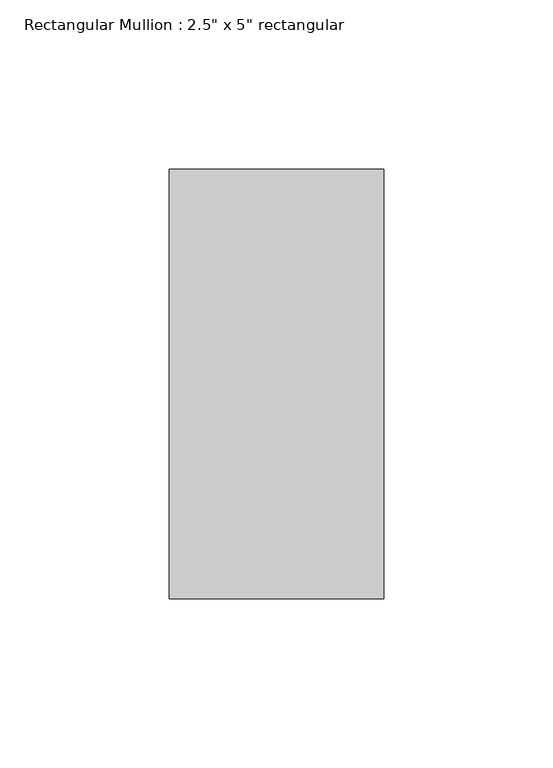
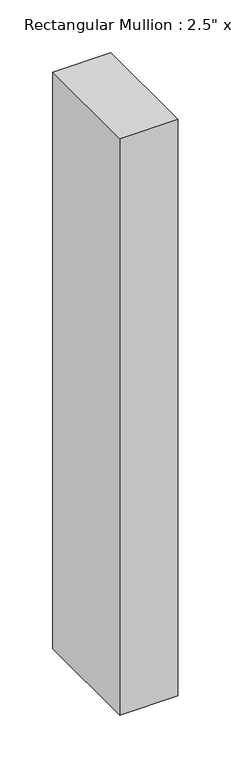
"""IFC4 building model written with IfcOpenShell, lengths in millimetres: member geometry."""

from ifc_helpers import new_model, si_unit, frame, origin, place, context, project, spatial, polyline, outline, extrude, source, transform, mapped, element, save


def member_c33c434a(model_context):
    return source(origin(), model_context, "Body", "SweptSolid", [
        extrude(outline(polyline([(0.0, 63.5), (0.0, -63.5), (-63.5, -63.5), (-63.5, 63.5), (0.0, 63.5)])), frame((0.0, 0.0, -666.75), z_axis=(0.0, 0.0, 1.0), x_axis=(1.0, 0.0, 0.0)), (0.0, 0.0, 1.0), 666.75),
    ])


if __name__ == "__main__":
    model = new_model("IFC4")
    model_context = context("Model", 3, world=origin())
    ifc_project = project(units=[si_unit("LENGTHUNIT", "METRE", prefix="MILLI")], contexts=[model_context])
    site = spatial("IfcSite", under=ifc_project)
    building = spatial("IfcBuilding", under=site)
    placement = place(None, origin())
    member_shape = member_c33c434a(model_context)
    element("IfcMember", 1, ObjectType="Rectangular Mullion : 2.5\" x 5\" rectangular", at=placement, inside=building, context=model_context, shape_type="MappedRepresentation", body=[
        mapped(member_shape, transform((0.0, 0.0, 0.0), x_axis=(1.0, 0.0, 0.0), y_axis=(0.0, 1.0, 0.0), z_axis=(0.0, 0.0, 1.0))),
    ])
    save(model, "model.ifc")

# Revit data of these elements
# Type "Rectangular Mullion : 2.5\" x 5\" rectangular"
#   built-in parameter 1007304 = 0.416667 (stored number, unit not read)
#   built-in parameter 1007301 = 0.104167 (stored number, unit not read)
#   built-in parameter 1007300 = 0.104167 (stored number, unit not read)
